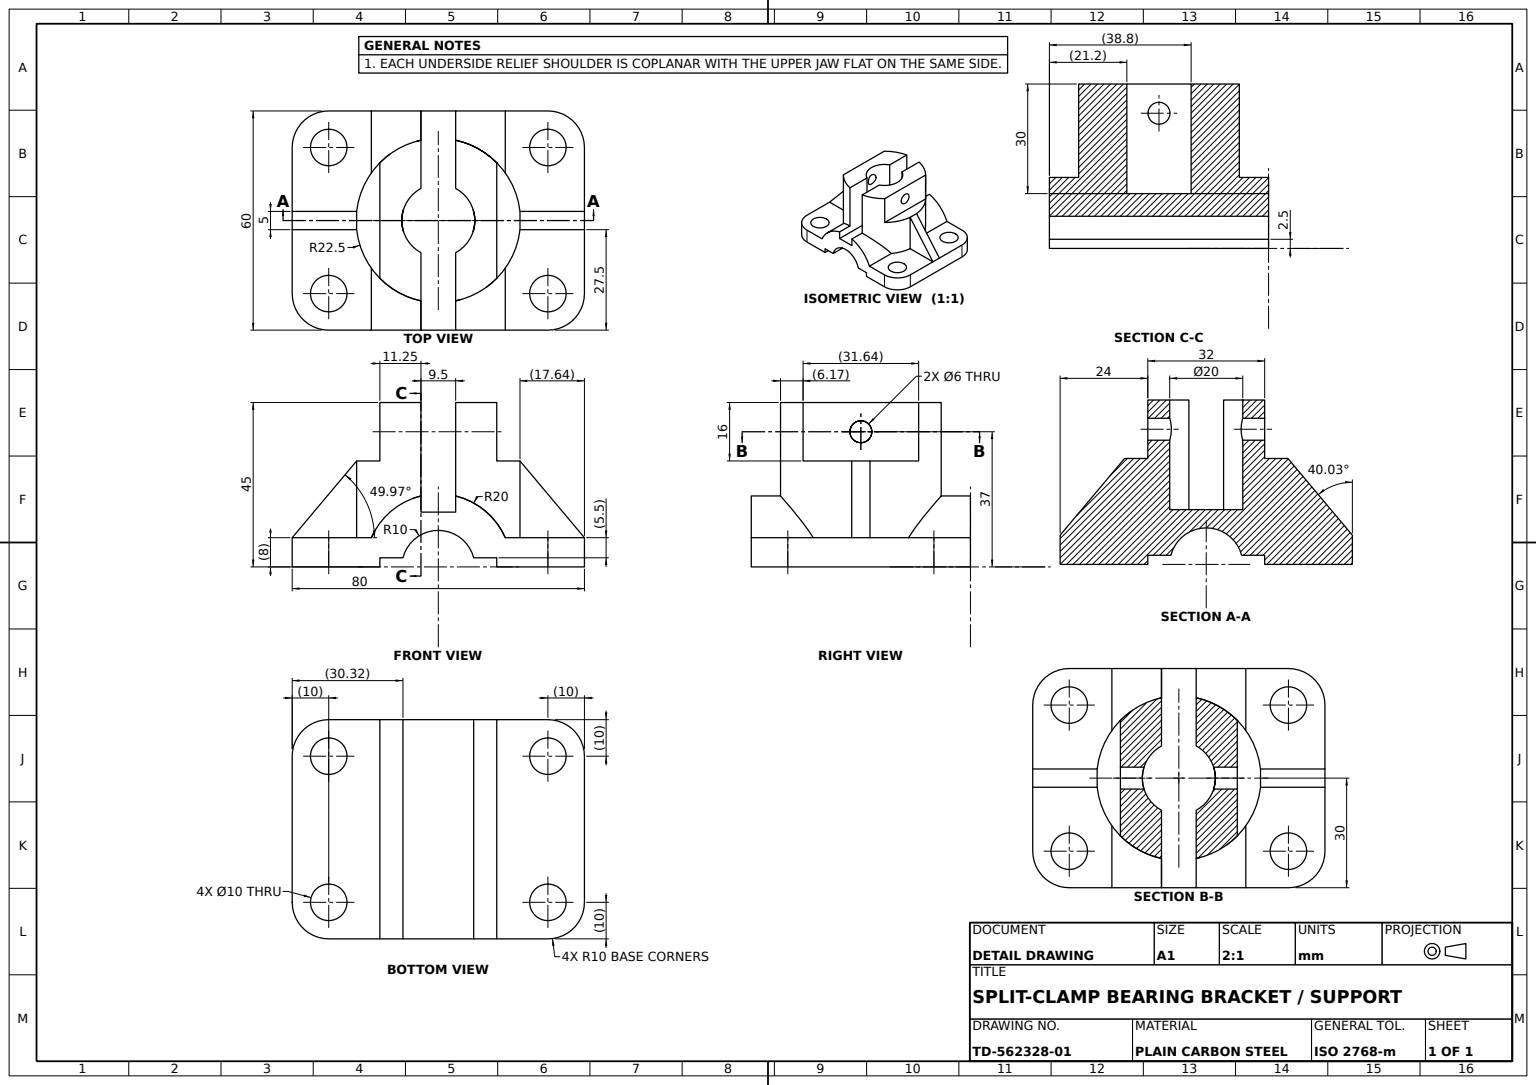
from build123d import *

# Parameters (mm, degrees)
BASE_BODY_DEPTH             = 60
VERTICAL_BOSS_SKETCH_R      = 22.5
VERTICAL_BOSS_40_DEPTH      = 38
BASE_HALF_BORE_SKETCH_R     = 10
BASE_HALF_BORE_20_DEPTH     = 60
BASE_CORNER_FILLETS_R10_R   = 10
MOUNTING_HOLES_SKETCH_R     = 5
MOUNTING_HOLES_4X_10_DEPTH  = 60
RIB_PROFILE_CUT_DEPTH       = 30
BOSS_UPPER_BORE_CUT_DEPTH   = 16
BOSS_LOWER_BORE_SKETCH_R    = 3
BOSS_LOWER_BORE_CUT_DEPTH   = 94.600213787
CLAMP_LUG_X62_SKETCH_W      = 5
CLAMP_LUG_X62_SKETCH_H      = 21
CLAMP_LUG_X62_DEPTH         = 18
LUG_X62_HOLE_CUT_DEPTH      = 98.37171055
LUG_X62_HOLE_CUT_DEPTH_BACK = 18
CLAMP_LUG_X18_SKETCH_W      = 5
CLAMP_LUG_X18_SKETCH_H      = 21
CLAMP_LUG_X18_DEPTH         = 18
LUG_X18_HOLE_CUT_DEPTH      = 98.37171055
LUG_X18_HOLE_CUT_DEPTH_BACK = 18


with BuildPart() as part:
    # Base Profile Sketch → Base Body (new body)
    with BuildSketch(Plane.XY):
        with BuildLine():
            Line((0, 0), (0, 8))
            Line((0, 8), (21.66969722, 8))
            ThreePointArc((21.66969722, 8), (40, 20), (58.33030278, 8))
            Line((58.33030278, 8), (80, 8))
            Line((80, 8), (80, 0))
            Line((80, 0), (56, 0))
            Line((56, 0), (56, 2.5))
            Line((56, 2.5), (49.682458366, 2.5))
            ThreePointArc((49.682458366, 2.5), (40, 10), (30.317541634, 2.5))
            Line((30.317541634, 2.5), (24, 2.5))
            Line((24, 2.5), (24, 0))
            Line((24, 0), (0, 0))
        make_face()
    extrude(amount=-BASE_BODY_DEPTH)

    # Vertical Boss Sketch → Vertical Boss Ø40 (add)
    with BuildSketch(Plane(origin=(0, 45, 0), x_dir=(1, 0, 0), z_dir=(0, 1, 0))):
        with Locations(Location((40, 30, 0), (0, 0, 270))):
            Circle(VERTICAL_BOSS_SKETCH_R)
    extrude(amount=-VERTICAL_BOSS_40_DEPTH)

    # Base Half Bore Sketch → Base Half Bore Ø20 (cut)
    with BuildSketch(Plane.XY):
        with Locations((40, 0)):
            Circle(BASE_HALF_BORE_SKETCH_R)
    extrude(amount=-BASE_HALF_BORE_20_DEPTH, mode=Mode.SUBTRACT)

    # Base Corner Fillets R10
    base_corner_fillets_r10_edges = [part.edges().sort_by_distance(p)[0] for p in [
        (0, 4, 0),
        (80, 4, 0),
        (80, 4, -60),
        (0, 4, -60),
    ]]
    fillet(base_corner_fillets_r10_edges, radius=BASE_CORNER_FILLETS_R10_R)

    # Mounting Holes Sketch → Mounting Holes 4xØ10 (cut)
    with BuildSketch(Plane(origin=(0, 8, 0), x_dir=(1, 0, 0), z_dir=(0, 1, 0))):
        with Locations(Location((70, 50, 0), (0, 0, 270))):
            Circle(MOUNTING_HOLES_SKETCH_R)
        with Locations(Location((70, 10, 0), (0, 0, 270))):
            Circle(MOUNTING_HOLES_SKETCH_R)
        with Locations(Location((10, 10, 0), (0, 0, 270))):
            Circle(MOUNTING_HOLES_SKETCH_R)
        with Locations(Location((10, 50, 0), (0, 0, 270))):
            Circle(MOUNTING_HOLES_SKETCH_R)
    extrude(amount=-MOUNTING_HOLES_4X_10_DEPTH, mode=Mode.SUBTRACT)

    # Rib Profile Sketch → Rib Profile Cut (cut)
    with BuildSketch(Plane(origin=(0, 45, 0), x_dir=(1, 0, 0), z_dir=(0, 1, 0))):
        with BuildLine():
            Line((35.25, 38.799857953), (35.25, 60))
            Line((35.25, 60), (44.75, 60))
            Line((44.75, 60), (44.75, 38.799857953))
            ThreePointArc((44.75, 38.799857953), (50, 30), (44.75, 21.200142047))
            Line((44.75, 21.200142047), (44.75, 0))
            Line((44.75, 0), (35.25, 0))
            Line((35.25, 0), (35.25, 21.200142047))
            ThreePointArc((35.25, 21.200142047), (30, 30), (35.25, 38.799857953))
        make_face()
    extrude(amount=-RIB_PROFILE_CUT_DEPTH, mode=Mode.SUBTRACT)

    # Boss Upper Bore Sketch → Boss Upper Bore Cut (cut)
    with BuildSketch(Plane(origin=(0, 45, 0), x_dir=(1, 0, 0), z_dir=(0, 1, 0))):
        with BuildLine():
            Line((56, 14.18070798), (56, 45.81929202))
            ThreePointArc((56, 45.81929202), (62.5, 30), (56, 14.18070798))
        make_face()
        with BuildLine():
            Line((24, 14.18070798), (24, 45.81929202))
            ThreePointArc((24, 45.81929202), (17.5, 30), (24, 14.18070798))
        make_face()
    extrude(amount=-BOSS_UPPER_BORE_CUT_DEPTH, mode=Mode.SUBTRACT)

    # Boss Lower Bore Sketch → Boss Lower Bore Cut (cut, through all)
    with BuildSketch(Plane(origin=(56, 0, 0), x_dir=(0, 0, -1), z_dir=(1, 0, 0))):
        with Locations((30, 37)):
            Circle(BOSS_LOWER_BORE_SKETCH_R)
    extrude(amount=-BOSS_LOWER_BORE_CUT_DEPTH, mode=Mode.SUBTRACT)

    # Clamp Lug X62 Sketch → Clamp Lug X62 (add)
    with BuildSketch(Plane(origin=(62, 0, 0), x_dir=(0, 0, -1), z_dir=(1, 0, 0))):
        with Locations((30, 18.5)):
            Rectangle(CLAMP_LUG_X62_SKETCH_W, CLAMP_LUG_X62_SKETCH_H)
    extrude(amount=CLAMP_LUG_X62_DEPTH)

    # Lug X62 Hole Sketch → Lug X62 Hole Cut (cut, two sides: drawn at the far end of the back side and taken through both)
    with BuildSketch(Plane.XY.offset(-27.5).offset(-LUG_X62_HOLE_CUT_DEPTH_BACK)):
        Polygon((80, 29), (62.360679775, 29), (80, 8), align=None)
    extrude(amount=LUG_X62_HOLE_CUT_DEPTH + LUG_X62_HOLE_CUT_DEPTH_BACK, mode=Mode.SUBTRACT)

    # Clamp Lug X18 Sketch → Clamp Lug X18 (add)
    with BuildSketch(Plane(origin=(18, 0, 0), x_dir=(0, 0, -1), z_dir=(1, 0, 0))):
        with Locations((30, 18.5)):
            Rectangle(CLAMP_LUG_X18_SKETCH_W, CLAMP_LUG_X18_SKETCH_H)
    extrude(amount=-CLAMP_LUG_X18_DEPTH)

    # Lug X18 Hole Sketch → Lug X18 Hole Cut (cut, two sides: drawn at the far end of the back side and taken through both)
    with BuildSketch(Plane(origin=(0, 0, -32.5), x_dir=(-1, 0, 0), z_dir=(0, 0, -1)).offset(-LUG_X18_HOLE_CUT_DEPTH_BACK)):
        Polygon((0, 29), (-17.639320225, 29), (0, 8), align=None)
    extrude(amount=LUG_X18_HOLE_CUT_DEPTH + LUG_X18_HOLE_CUT_DEPTH_BACK, mode=Mode.SUBTRACT)


solid = part.part
